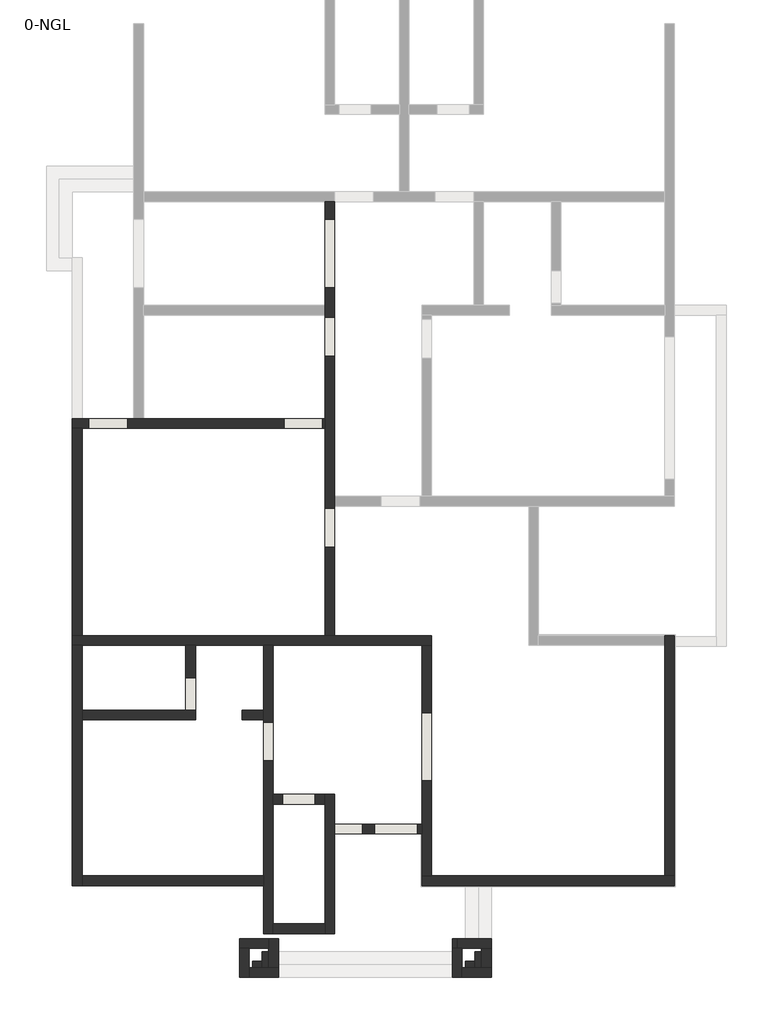
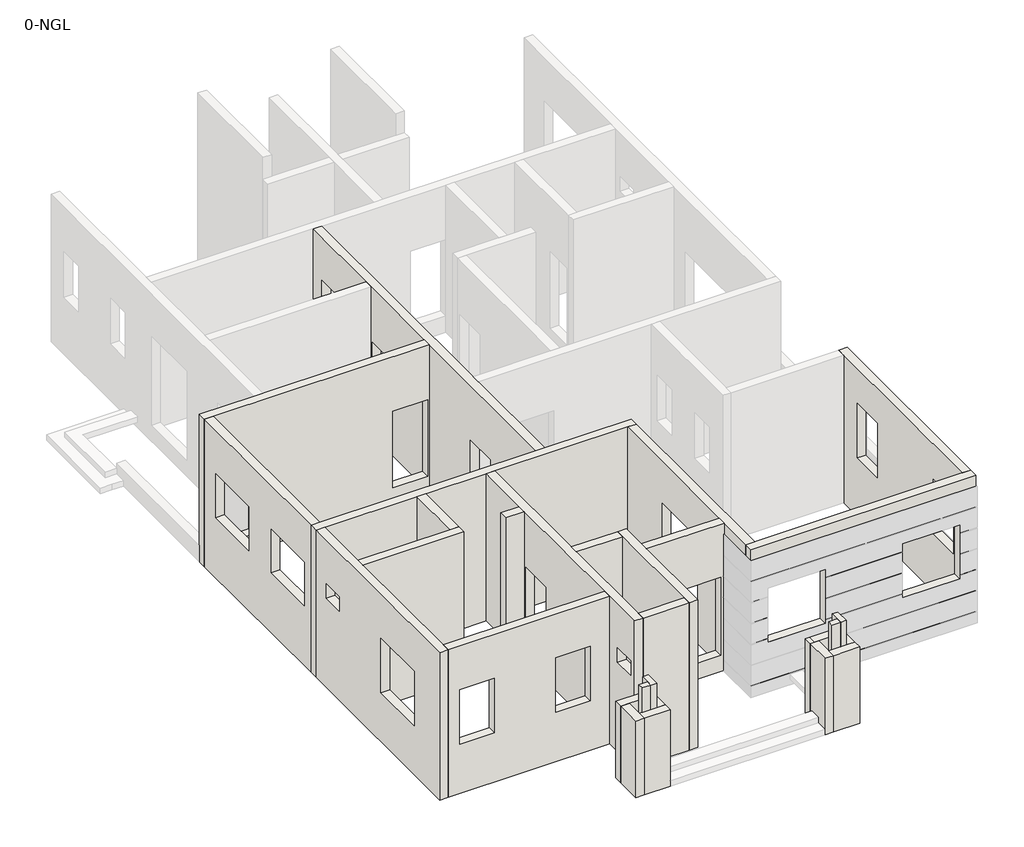
# One storey, part 1 of 2: 31 walls.
"""IFC4 building model written with IfcOpenShell, lengths in millimetres."""

from ifc_helpers import new_model, si_unit, frame, origin, origin_with_axes, place, context, project, spatial, polyline, outline, extrude, faceted_brep, element, save

model = new_model("IFC4")

# Units and contexts
model_context = context("Model", 3, world=origin())
ifc_project = project(units=[si_unit("LENGTHUNIT", "METRE", prefix="MILLI")], contexts=[model_context])

# Site, building, storey
site = spatial("IfcSite", under=ifc_project)
building = spatial("IfcBuilding", under=site)
storey = spatial("IfcBuildingStorey", under=building, Name="0-NGL", Elevation=0.0)

# Walls
placement = place(None, origin())
element("IfcWall", 1, ObjectType="150mm wall", at=placement, inside=storey, context=model_context, shape_type="Brep", body=[
    faceted_brep([(-1711.7953966, -12624.1929163, 0.0), (-1711.7953966, -12849.1929163, 0.0), (-1711.7953966, -12999.1929163, 0.0), (-1711.7953966, -12999.1929163, 2775.0), (-1711.7953966, -12849.1929163, 2775.0), (-1711.7953966, -12624.1929163, 2775.0), (-1561.7953966, -12624.1929163, 0.0), (-1561.7953966, -12624.1929163, 2775.0), (-1561.7953966, -12999.1929163, 2775.0), (-1561.7953966, -12999.1929163, 0.0)], [[[0, 1, 2, 3, 4, 5]], [[6, 7, 8, 9]], [[2, 1, 0, 6, 9]], [[5, 4, 3, 8, 7]], [[0, 5, 7, 6]], [[3, 2, 9, 8]]]),
])
element("IfcWall", 2, ObjectType="150mm wall", at=placement, inside=storey, context=model_context, shape_type="SweptSolid", body=[
    extrude(outline(polyline([(-1936.7953966, -12849.1929163), (-1711.7953966, -12849.1929163), (-1711.7953966, -12999.1929163), (-1936.7953966, -12999.1929163), (-1936.7953966, -12849.1929163)])), origin_with_axes(), (0.0, 0.0, 1.0), 2775.0),
])
element("IfcWall", 3, ObjectType="150mm wall", at=placement, inside=storey, context=model_context, shape_type="Brep", body=[
    faceted_brep([(3218.2046034, -12624.1929163, 0.0), (3218.2046034, -12849.1929163, 0.0), (3218.2046034, -12999.1929163, 0.0), (3218.2046034, -12999.1929163, 2775.0), (3218.2046034, -12849.1929163, 2775.0), (3218.2046034, -12624.1929163, 2775.0), (3368.2046034, -12624.1929163, 0.0), (3368.2046034, -12624.1929163, 2775.0), (3368.2046034, -12999.1929163, 2775.0), (3368.2046034, -12999.1929163, 0.0)], [[[0, 1, 2, 3, 4, 5]], [[6, 7, 8, 9]], [[2, 1, 0, 6, 9]], [[5, 4, 3, 8, 7]], [[0, 5, 7, 6]], [[3, 2, 9, 8]]]),
])
element("IfcWall", 4, ObjectType="150mm wall", at=placement, inside=storey, context=model_context, shape_type="SweptSolid", body=[
    extrude(outline(polyline([(2993.2046034, -12849.1929163), (3218.2046034, -12849.1929163), (3218.2046034, -12999.1929163), (2993.2046034, -12999.1929163), (2993.2046034, -12849.1929163)])), origin_with_axes(), (0.0, 0.0, 1.0), 2775.0),
])
element("IfcWall", 5, ObjectType="225 wall", at=placement, inside=storey, context=model_context, shape_type="Brep", body=[
    faceted_brep([(7838.2046034, -10871.6929163, 0.0), (7613.2046034, -10871.6929163, 0.0), (2213.2046034, -10871.6929163, 0.0), (1988.2046034, -10871.6929163, 0.0), (1988.2046034, -10871.6929163, 4050.0), (2213.2046034, -10871.6929163, 4050.0), (7613.2046034, -10871.6929163, 4050.0), (7838.2046034, -10871.6929163, 4050.0), (3913.2046034, -10871.6929163, 2850.0), (2413.2046034, -10871.6929163, 2850.0), (2413.2046034, -10871.6929163, 1350.0), (3913.2046034, -10871.6929163, 1350.0), (7413.2046034, -10871.6929163, 2850.0), (5913.2046034, -10871.6929163, 2850.0), (5913.2046034, -10871.6929163, 1350.0), (7413.2046034, -10871.6929163, 1350.0), (7838.2046034, -11096.6929163, 0.0), (7838.2046034, -11096.6929163, 4050.0), (1988.2046034, -11096.6929163, 4050.0), (1988.2046034, -11096.6929163, 0.0), (3913.2046034, -11096.6929163, 2850.0), (3913.2046034, -11096.6929163, 1350.0), (2413.2046034, -11096.6929163, 1350.0), (2413.2046034, -11096.6929163, 2850.0), (7413.2046034, -11096.6929163, 2850.0), (7413.2046034, -11096.6929163, 1350.0), (5913.2046034, -11096.6929163, 1350.0), (5913.2046034, -11096.6929163, 2850.0)], [[[0, 1, 2, 3, 4, 5, 6, 7], [8, 9, 10, 11], [12, 13, 14, 15]], [[16, 17, 18, 19], [20, 21, 22, 23], [24, 25, 26, 27]], [[3, 2, 1, 0, 16, 19]], [[7, 6, 5, 4, 18, 17]], [[0, 7, 17, 16]], [[4, 3, 19, 18]], [[21, 20, 8, 11]], [[22, 21, 11, 10]], [[23, 22, 10, 9]], [[20, 23, 9, 8]], [[25, 24, 12, 15]], [[26, 25, 15, 14]], [[27, 26, 14, 13]], [[24, 27, 13, 12]]]),
])
element("IfcWall", 6, ObjectType="225 wall", at=placement, inside=storey, context=model_context, shape_type="Brep", body=[
    faceted_brep([(-5886.7953966, -11096.6929163, 0.0), (-5886.7953966, -10871.6929163, 0.0), (-5886.7953966, -7259.1929163, 0.0), (-5886.7953966, -7034.1929163, 0.0), (-5886.7953966, -5534.1929163, 0.0), (-5886.7953966, -5534.1929163, 4050.0), (-5886.7953966, -7034.1929163, 4050.0), (-5886.7953966, -7259.1929163, 4050.0), (-5886.7953966, -10871.6929163, 4050.0), (-5886.7953966, -11096.6929163, 4050.0), (-5886.7953966, -6584.1929163, 2850.0), (-5886.7953966, -5984.1929163, 2850.0), (-5886.7953966, -5984.1929163, 2450.0), (-5886.7953966, -6584.1929163, 2450.0), (-5886.7953966, -8459.1929163, 2850.0), (-5886.7953966, -8459.1929163, 1350.0), (-5886.7953966, -9959.1929163, 1350.0), (-5886.7953966, -9959.1929163, 2850.0), (-6111.7953966, -11096.6929163, 0.0), (-6111.7953966, -11096.6929163, 4050.0), (-6111.7953966, -5534.1929163, 4050.0), (-6111.7953966, -5534.1929163, 0.0), (-6111.7953966, -6584.1929163, 2850.0), (-6111.7953966, -6584.1929163, 2450.0), (-6111.7953966, -5984.1929163, 2450.0), (-6111.7953966, -5984.1929163, 2850.0), (-6111.7953966, -8459.1929163, 2850.0), (-6111.7953966, -9959.1929163, 2850.0), (-6111.7953966, -9959.1929163, 1350.0), (-6111.7953966, -8459.1929163, 1350.0)], [[[0, 1, 2, 3, 4, 5, 6, 7, 8, 9], [10, 11, 12, 13], [14, 15, 16, 17]], [[18, 19, 20, 21], [22, 23, 24, 25], [26, 27, 28, 29]], [[4, 3, 2, 1, 0, 18, 21]], [[9, 8, 7, 6, 5, 20, 19]], [[5, 4, 21, 20]], [[0, 9, 19, 18]], [[23, 22, 10, 13]], [[24, 23, 13, 12]], [[25, 24, 12, 11]], [[22, 25, 11, 10]], [[15, 14, 26, 29]], [[16, 15, 29, 28]], [[17, 16, 28, 27]], [[14, 17, 27, 26]]]),
])
element("IfcWall", 7, ObjectType="225 wall", at=placement, inside=storey, context=model_context, shape_type="Brep", body=[
    faceted_brep([(-1461.7953966, -12209.1929163, 4050.0), (-1461.7953966, -12209.1929163, 0.0), (-1461.7953966, -11984.1929163, 0.0), (-1461.7953966, -9209.1929163, 0.0), (-1461.7953966, -8984.1929163, 0.0), (-1461.7953966, -5534.1929163, 0.0), (-1461.7953966, -5534.1929163, 4050.0), (-1461.7953966, -8984.1929163, 4050.0), (-1461.7953966, -9209.1929163, 4050.0), (-1461.7953966, -11984.1929163, 4050.0), (-1461.7953966, -7309.1929163, 450.0), (-1461.7953966, -8209.1929163, 450.0), (-1461.7953966, -8209.1929163, 2550.0), (-1461.7953966, -7309.1929163, 2550.0), (-1461.7953966, -11444.1929163, 2850.0), (-1461.7953966, -11444.1929163, 2450.0), (-1461.7953966, -12044.1929163, 2450.0), (-1461.7953966, -12044.1929163, 2850.0), (-1686.7953966, -12209.1929163, 0.0), (-1686.7953966, -12209.1929163, 4050.0), (-1686.7953966, -11096.6929163, 4050.0), (-1686.7953966, -10871.6929163, 4050.0), (-1686.7953966, -7259.1929163, 4050.0), (-1686.7953966, -7034.1929163, 4050.0), (-1686.7953966, -5534.1929163, 4050.0), (-1686.7953966, -5534.1929163, 0.0), (-1686.7953966, -7034.1929163, 0.0), (-1686.7953966, -7259.1929163, 0.0), (-1686.7953966, -10871.6929163, 0.0), (-1686.7953966, -11096.6929163, 0.0), (-1686.7953966, -7309.1929163, 450.0), (-1686.7953966, -7309.1929163, 2550.0), (-1686.7953966, -8209.1929163, 2550.0), (-1686.7953966, -8209.1929163, 450.0), (-1686.7953966, -11444.1929163, 2850.0), (-1686.7953966, -12044.1929163, 2850.0), (-1686.7953966, -12044.1929163, 2450.0), (-1686.7953966, -11444.1929163, 2450.0)], [[[0, 1, 2, 3, 4, 5, 6, 7, 8, 9], [10, 11, 12, 13], [14, 15, 16, 17]], [[18, 19, 20, 21, 22, 23, 24, 25, 26, 27, 28, 29], [30, 31, 32, 33], [34, 35, 36, 37]], [[5, 4, 3, 2, 1, 18, 29, 28, 27, 26, 25]], [[0, 9, 8, 7, 6, 24, 23, 22, 21, 20, 19]], [[6, 5, 25, 24]], [[31, 30, 10, 13]], [[32, 31, 13, 12]], [[33, 32, 12, 11]], [[30, 33, 11, 10]], [[15, 14, 34, 37]], [[16, 15, 37, 36]], [[17, 16, 36, 35]], [[14, 17, 35, 34]], [[0, 19, 18, 1]]]),
])
element("IfcWall", 8, ObjectType="225 wall", at=placement, inside=storey, context=model_context, shape_type="Brep", body=[
    faceted_brep([(-6111.7953966, -509.1929163, 4050.0), (-6111.7953966, -509.1929163, 0.0), (-5886.7953966, -509.1929163, 0.0), (-261.7953966, -509.1929163, 0.0), (-261.7953966, -509.1929163, 4050.0), (-5886.7953966, -509.1929163, 4050.0), (-4836.7953966, -509.1929163, 450.0), (-5736.7953966, -509.1929163, 450.0), (-5736.7953966, -509.1929163, 2550.0), (-4836.7953966, -509.1929163, 2550.0), (-311.7953966, -509.1929163, 450.0), (-1211.7953966, -509.1929163, 450.0), (-1211.7953966, -509.1929163, 2550.0), (-311.7953966, -509.1929163, 2550.0), (-6111.7953966, -284.1929163, 0.0), (-6111.7953966, -284.1929163, 450.0), (-6111.7953966, -284.1929163, 3450.0), (-6111.7953966, -284.1929163, 4042.0), (-6111.7953966, -284.1929163, 4050.0), (-4686.7953966, -284.1929163, 4050.0), (-4461.7953966, -284.1929163, 4050.0), (-261.7953966, -284.1929163, 4050.0), (-261.7953966, -284.1929163, 0.0), (-4461.7953966, -284.1929163, 0.0), (-4686.7953966, -284.1929163, 0.0), (-5886.7953966, -284.1929163, 0.0), (-4836.7953966, -284.1929163, 450.0), (-4836.7953966, -284.1929163, 2550.0), (-5736.7953966, -284.1929163, 2550.0), (-5736.7953966, -284.1929163, 450.0), (-311.7953966, -284.1929163, 450.0), (-311.7953966, -284.1929163, 2550.0), (-1211.7953966, -284.1929163, 2550.0), (-1211.7953966, -284.1929163, 450.0)], [[[0, 1, 2, 3, 4, 5], [6, 7, 8, 9], [10, 11, 12, 13]], [[14, 15, 16, 17, 18, 19, 20, 21, 22, 23, 24, 25], [26, 27, 28, 29], [30, 31, 32, 33]], [[3, 2, 1, 14, 25, 24, 23, 22]], [[0, 5, 4, 21, 20, 19, 18]], [[4, 3, 22, 21]], [[27, 26, 6, 9]], [[28, 27, 9, 8]], [[29, 28, 8, 7]], [[26, 29, 7, 6]], [[31, 30, 10, 13]], [[32, 31, 13, 12]], [[33, 32, 12, 11]], [[30, 33, 11, 10]], [[0, 18, 17, 16, 15, 14, 1]]]),
])
element("IfcWall", 9, ObjectType="225 wall", at=placement, inside=storey, context=model_context, shape_type="Brep", body=[
    faceted_brep([(7838.2046034, -10871.6929163, 0.0), (7838.2046034, -5559.1929163, 0.0), (7838.2046034, -5334.1929163, 0.0), (7838.2046034, -5309.1929163, 0.0), (7838.2046034, -5309.1929163, 3450.0), (7838.2046034, -5309.1929163, 4050.0), (7838.2046034, -10871.6929163, 4050.0), (7838.2046034, -9571.6929163, 3090.0), (7838.2046034, -9571.6929163, 1590.0), (7838.2046034, -10471.6929163, 1590.0), (7838.2046034, -10471.6929163, 3090.0), (7838.2046034, -6134.1929163, 3090.0), (7838.2046034, -6134.1929163, 1590.0), (7838.2046034, -7034.1929163, 1590.0), (7838.2046034, -7034.1929163, 3090.0), (7613.2046034, -10871.6929163, 0.0), (7613.2046034, -10871.6929163, 4050.0), (7613.2046034, -5534.1929163, 4050.0), (7613.2046034, -5309.1929163, 4050.0), (7613.2046034, -5309.1929163, 0.0), (7613.2046034, -5534.1929163, 0.0), (7613.2046034, -9571.6929163, 3090.0), (7613.2046034, -10471.6929163, 3090.0), (7613.2046034, -10471.6929163, 1590.0), (7613.2046034, -9571.6929163, 1590.0), (7613.2046034, -6134.1929163, 3090.0), (7613.2046034, -7034.1929163, 3090.0), (7613.2046034, -7034.1929163, 1590.0), (7613.2046034, -6134.1929163, 1590.0)], [[[0, 1, 2, 3, 4, 5, 6], [7, 8, 9, 10], [11, 12, 13, 14]], [[15, 16, 17, 18, 19, 20], [21, 22, 23, 24], [25, 26, 27, 28]], [[3, 2, 1, 0, 15, 20, 19]], [[6, 5, 18, 17, 16]], [[0, 6, 16, 15]], [[8, 7, 21, 24]], [[9, 8, 24, 23]], [[10, 9, 23, 22]], [[7, 10, 22, 21]], [[12, 11, 25, 28]], [[13, 12, 28, 27]], [[14, 13, 27, 26]], [[11, 14, 26, 25]], [[3, 19, 18, 5, 4]]]),
])
element("IfcWall", 10, ObjectType="225 wall", at=placement, inside=storey, context=model_context, shape_type="Brep", body=[
    faceted_brep([(-6111.7953966, -5534.1929163, 0.0), (-5886.7953966, -5534.1929163, 0.0), (-3486.7953966, -5534.1929163, 0.0), (-3261.7953966, -5534.1929163, 0.0), (-1686.7953966, -5534.1929163, 0.0), (-1461.7953966, -5534.1929163, 0.0), (1988.2046034, -5534.1929163, 0.0), (2213.2046034, -5534.1929163, 0.0), (2213.2046034, -5534.1929163, 4050.0), (1988.2046034, -5534.1929163, 4050.0), (-1461.7953966, -5534.1929163, 4050.0), (-1686.7953966, -5534.1929163, 4050.0), (-3261.7953966, -5534.1929163, 4050.0), (-3486.7953966, -5534.1929163, 4050.0), (-5886.7953966, -5534.1929163, 4050.0), (-6111.7953966, -5534.1929163, 4050.0), (-6111.7953966, -5309.1929163, 0.0), (-6111.7953966, -5309.1929163, 4050.0), (-5886.7953966, -5309.1929163, 4050.0), (-261.7953966, -5309.1929163, 4050.0), (-36.7953966, -5309.1929163, 4050.0), (2213.2046034, -5309.1929163, 4050.0), (2213.2046034, -5309.1929163, 0.0), (-36.7953966, -5309.1929163, 0.0), (-261.7953966, -5309.1929163, 0.0), (-5886.7953966, -5309.1929163, 0.0)], [[[0, 1, 2, 3, 4, 5, 6, 7, 8, 9, 10, 11, 12, 13, 14, 15]], [[16, 17, 18, 19, 20, 21, 22, 23, 24, 25]], [[7, 6, 5, 4, 3, 2, 1, 0, 16, 25, 24, 23, 22]], [[15, 14, 13, 12, 11, 10, 9, 8, 21, 20, 19, 18, 17]], [[0, 15, 17, 16]], [[8, 7, 22, 21]]]),
])
element("IfcWall", 11, ObjectType="225 wall", at=placement, inside=storey, context=model_context, shape_type="SweptSolid", body=[
    extrude(outline(polyline([(-5309.1929163, 0.0), (-5309.1929163, 4050.0), (-509.1929163, 4050.0), (-509.1929163, 0.0), (-5309.1929163, 0.0)]), holes=[polyline([(-1009.1929163, 2850.0), (-2509.1929163, 2850.0), (-2509.1929163, 1650.0), (-1009.1929163, 1650.0), (-1009.1929163, 2850.0)]), polyline([(-3509.1929163, 2850.0), (-5009.1929163, 2850.0), (-5009.1929163, 1650.0), (-3509.1929163, 1650.0), (-3509.1929163, 2850.0)])]), frame((-6111.7953966, 0.0, 0.0), z_axis=(1.0, 0.0, 0.0), x_axis=(0.0, 1.0, 0.0)), (0.0, 0.0, 1.0), 225.0),
])
element("IfcWall", 12, ObjectType="225 wall", at=placement, inside=storey, context=model_context, shape_type="Brep", body=[
    faceted_brep([(-5886.7953966, -7259.1929163, 0.0), (-3261.7953966, -7259.1929163, 0.0), (-3261.7953966, -7259.1929163, 4050.0), (-5886.7953966, -7259.1929163, 4050.0), (-5886.7953966, -7034.1929163, 0.0), (-5886.7953966, -7034.1929163, 4050.0), (-3486.7953966, -7034.1929163, 4050.0), (-3261.7953966, -7034.1929163, 4050.0), (-3261.7953966, -7034.1929163, 2550.0), (-3261.7953966, -7034.1929163, 450.0), (-3261.7953966, -7034.1929163, 0.0), (-3486.7953966, -7034.1929163, 0.0)], [[[0, 1, 2, 3]], [[4, 5, 6, 7, 8, 9, 10, 11]], [[1, 0, 4, 11, 10]], [[2, 1, 10, 9, 8, 7]], [[3, 2, 7, 6, 5]], [[0, 3, 5, 4]]]),
])
element("IfcWall", 13, ObjectType="225 wall", at=placement, inside=storey, context=model_context, shape_type="SweptSolid", body=[
    extrude(outline(polyline([(0.0, -5886.7953966), (0.0, -1686.7953966), (4050.0, -1686.7953966), (4050.0, -5886.7953966), (0.0, -5886.7953966)]), holes=[polyline([(2850.0, -2186.7953966), (1350.0, -2186.7953966), (1350.0, -3086.7953966), (2850.0, -3086.7953966), (2850.0, -2186.7953966)]), polyline([(2850.0, -4686.7953966), (1350.0, -4686.7953966), (1350.0, -5586.7953966), (2850.0, -5586.7953966), (2850.0, -4686.7953966)])]), frame((0.0, -11096.6929163, 0.0), z_axis=(0.0, 1.0, 0.0), x_axis=(0.0, 0.0, 1.0)), (0.0, 0.0, 1.0), 225.0),
])
element("IfcWall", 14, ObjectType="225 wall", at=placement, inside=storey, context=model_context, shape_type="Brep", body=[
    faceted_brep([(2213.2046034, -10871.6929163, 0.0), (2213.2046034, -5534.1929163, 0.0), (2213.2046034, -5534.1929163, 4050.0), (2213.2046034, -10871.6929163, 4050.0), (2213.2046034, -7091.6929163, 450.0), (2213.2046034, -8671.6929163, 450.0), (2213.2046034, -8671.6929163, 2890.0), (2213.2046034, -7091.6929163, 2890.0), (1988.2046034, -10871.6929163, 0.0), (1988.2046034, -10871.6929163, 4050.0), (1988.2046034, -9896.6929163, 4050.0), (1988.2046034, -9671.6929163, 4050.0), (1988.2046034, -5534.1929163, 4050.0), (1988.2046034, -5534.1929163, 0.0), (1988.2046034, -9671.6929163, 0.0), (1988.2046034, -9896.6929163, 0.0), (1988.2046034, -7091.6929163, 450.0), (1988.2046034, -7091.6929163, 2890.0), (1988.2046034, -8671.6929163, 2890.0), (1988.2046034, -8671.6929163, 450.0)], [[[0, 1, 2, 3], [4, 5, 6, 7]], [[8, 9, 10, 11, 12, 13, 14, 15], [16, 17, 18, 19]], [[1, 0, 8, 15, 14, 13]], [[3, 2, 12, 11, 10, 9]], [[0, 3, 9, 8]], [[17, 16, 4, 7]], [[18, 17, 7, 6]], [[19, 18, 6, 5]], [[16, 19, 5, 4]], [[2, 1, 13, 12]]]),
])
element("IfcWall", 15, ObjectType="225 wall", at=placement, inside=storey, context=model_context, shape_type="Brep", body=[
    faceted_brep([(-36.7953966, -5309.1929163, 0.0), (-36.7953966, -2309.1929163, 0.0), (-36.7953966, -2084.1929163, 0.0), (-36.7953966, 4740.8070837, 0.0), (-36.7953966, 4740.8070837, 450.0), (-36.7953966, 4740.8070837, 2550.0), (-36.7953966, 4740.8070837, 4050.0), (-36.7953966, -2084.1929163, 4050.0), (-36.7953966, -2309.1929163, 4050.0), (-36.7953966, -5309.1929163, 4050.0), (-36.7953966, -2359.1929163, 450.0), (-36.7953966, -3259.1929163, 450.0), (-36.7953966, -3259.1929163, 2550.0), (-36.7953966, -2359.1929163, 2550.0), (-36.7953966, 4330.8070837, 450.0), (-36.7953966, 2750.8070837, 450.0), (-36.7953966, 2750.8070837, 2890.0), (-36.7953966, 4330.8070837, 2890.0), (-36.7953966, 2065.8070837, 450.0), (-36.7953966, 1165.8070837, 450.0), (-36.7953966, 1165.8070837, 2550.0), (-36.7953966, 2065.8070837, 2550.0), (-261.7953966, -5309.1929163, 0.0), (-261.7953966, -5309.1929163, 4050.0), (-261.7953966, -509.1929163, 4050.0), (-261.7953966, -284.1929163, 4050.0), (-261.7953966, 2115.8070837, 4050.0), (-261.7953966, 2340.8070837, 4050.0), (-261.7953966, 4740.8070837, 4050.0), (-261.7953966, 4740.8070837, 0.0), (-261.7953966, 2340.8070837, 0.0), (-261.7953966, 2115.8070837, 0.0), (-261.7953966, -284.1929163, 0.0), (-261.7953966, -509.1929163, 0.0), (-261.7953966, -2359.1929163, 450.0), (-261.7953966, -2359.1929163, 2550.0), (-261.7953966, -3259.1929163, 2550.0), (-261.7953966, -3259.1929163, 450.0), (-261.7953966, 4330.8070837, 450.0), (-261.7953966, 4330.8070837, 2890.0), (-261.7953966, 2750.8070837, 2890.0), (-261.7953966, 2750.8070837, 450.0), (-261.7953966, 2065.8070837, 450.0), (-261.7953966, 2065.8070837, 2550.0), (-261.7953966, 1165.8070837, 2550.0), (-261.7953966, 1165.8070837, 450.0)], [[[0, 1, 2, 3, 4, 5, 6, 7, 8, 9], [10, 11, 12, 13], [14, 15, 16, 17], [18, 19, 20, 21]], [[22, 23, 24, 25, 26, 27, 28, 29, 30, 31, 32, 33], [34, 35, 36, 37], [38, 39, 40, 41], [42, 43, 44, 45]], [[3, 2, 1, 0, 22, 33, 32, 31, 30, 29]], [[9, 8, 7, 6, 28, 27, 26, 25, 24, 23]], [[6, 5, 4, 3, 29, 28]], [[0, 9, 23, 22]], [[35, 34, 10, 13]], [[36, 35, 13, 12]], [[37, 36, 12, 11]], [[34, 37, 11, 10]], [[39, 38, 14, 17]], [[40, 39, 17, 16]], [[41, 40, 16, 15]], [[38, 41, 15, 14]], [[43, 42, 18, 21]], [[44, 43, 21, 20]], [[45, 44, 20, 19]], [[42, 45, 19, 18]]]),
])
element("IfcWall", 16, ObjectType="225 wall", at=placement, inside=storey, context=model_context, shape_type="Brep", body=[
    faceted_brep([(-36.7953966, -12209.1929163, 0.0), (-36.7953966, -9896.6929163, 0.0), (-36.7953966, -9671.6929163, 0.0), (-36.7953966, -8984.1929163, 0.0), (-36.7953966, -8984.1929163, 4050.0), (-36.7953966, -9671.6929163, 4050.0), (-36.7953966, -9896.6929163, 4050.0), (-36.7953966, -12209.1929163, 4050.0), (-261.7953966, -8984.1929163, 0.0), (-261.7953966, -9209.1929163, 0.0), (-261.7953966, -11984.1929163, 0.0), (-261.7953966, -12209.1929163, 0.0), (-261.7953966, -12209.1929163, 4050.0), (-261.7953966, -11984.1929163, 4050.0), (-261.7953966, -9209.1929163, 4050.0), (-261.7953966, -8984.1929163, 4050.0)], [[[0, 1, 2, 3, 4, 5, 6, 7]], [[8, 9, 10, 11, 12, 13, 14, 15]], [[3, 2, 1, 0, 11, 10, 9, 8]], [[7, 6, 5, 4, 15, 14, 13, 12]], [[4, 3, 8, 15]], [[0, 7, 12, 11]]]),
])
element("IfcWall", 17, ObjectType="225 wall", at=placement, inside=storey, context=model_context, shape_type="SweptSolid", body=[
    extrude(outline(polyline([(0.0, -261.7953966), (4050.0, -261.7953966), (4050.0, -1461.7953966), (0.0, -1461.7953966), (0.0, -261.7953966)]), holes=[polyline([(450.0, -1236.7953966), (2550.0, -1236.7953966), (2550.0, -486.7953966), (450.0, -486.7953966), (450.0, -1236.7953966)])]), frame((0.0, -9209.1929163, 0.0), z_axis=(0.0, 1.0, 0.0), x_axis=(0.0, 0.0, 1.0)), (0.0, 0.0, 1.0), 225.0),
])
element("IfcWall", 18, ObjectType="225 wall", at=placement, inside=storey, context=model_context, shape_type="SweptSolid", body=[
    extrude(outline(polyline([(-1461.7953966, -11984.1929163), (-261.7953966, -11984.1929163), (-261.7953966, -12209.1929163), (-1461.7953966, -12209.1929163), (-1461.7953966, -11984.1929163)])), origin_with_axes(), (0.0, 0.0, 1.0), 4050.0),
])
element("IfcWall", 19, ObjectType="225 wall", at=placement, inside=storey, context=model_context, shape_type="SweptSolid", body=[
    extrude(outline(polyline([(0.0, -36.7953966), (0.0, 1988.2046034), (4050.0, 1988.2046034), (4050.0, -36.7953966), (2275.0, -36.7953966), (2275.0, 613.2046034), (1025.0, 613.2046034), (1025.0, -36.7953966), (0.0, -36.7953966)]), holes=[polyline([(450.0, 888.2046034), (2595.0, 888.2046034), (2595.0, 1888.2046034), (450.0, 1888.2046034), (450.0, 888.2046034)])]), frame((0.0, -9896.6929163, 0.0), z_axis=(0.0, 1.0, 0.0), x_axis=(0.0, 0.0, 1.0)), (0.0, 0.0, 1.0), 225.0),
])
element("IfcWall", 20, ObjectType="225 wall", at=placement, inside=storey, context=model_context, shape_type="SweptSolid", body=[
    extrude(outline(polyline([(-6284.1929163, 2550.0), (-7034.1929163, 2550.0), (-7034.1929163, 4050.0), (-5534.1929163, 4050.0), (-5534.1929163, 0.0), (-7034.1929163, 0.0), (-7034.1929163, 450.0), (-6284.1929163, 450.0), (-6284.1929163, 2550.0)])), frame((-3486.7953966, 0.0, 0.0), z_axis=(1.0, 0.0, 0.0), x_axis=(0.0, 1.0, 0.0)), (0.0, 0.0, 1.0), 225.0),
])
element("IfcWall", 21, ObjectType="225 wall", at=placement, inside=storey, context=model_context, shape_type="SweptSolid", body=[
    extrude(outline(polyline([(-1686.7953966, -7259.1929163), (-2174.2953966, -7259.1929163), (-2174.2953966, -7034.1929163), (-1686.7953966, -7034.1929163), (-1686.7953966, -7259.1929163)])), origin_with_axes(), (0.0, 0.0, 1.0), 4050.0),
])
element("IfcWall", 22, ObjectType="225 wall", at=placement, inside=storey, context=model_context, shape_type="Brep", body=[
    faceted_brep([(-2236.7953966, -12549.1929163, 0.0), (-2011.7953966, -12549.1929163, 0.0), (-1561.7953966, -12549.1929163, 0.0), (-1561.7953966, -12549.1929163, 2100.0), (-2011.7953966, -12549.1929163, 2100.0), (-2236.7953966, -12549.1929163, 2100.0), (-2236.7953966, -12324.1929163, 0.0), (-2236.7953966, -12324.1929163, 2100.0), (-1561.7953966, -12324.1929163, 2100.0), (-1561.7953966, -12324.1929163, 0.0)], [[[0, 1, 2, 3, 4, 5]], [[6, 7, 8, 9]], [[2, 1, 0, 6, 9]], [[5, 4, 3, 8, 7]], [[0, 5, 7, 6]], [[3, 2, 9, 8]]]),
])
element("IfcWall", 23, ObjectType="225 wall", at=placement, inside=storey, context=model_context, shape_type="Brep", body=[
    faceted_brep([(-2011.7953966, -13224.1929163, 0.0), (-2011.7953966, -12999.1929163, 0.0), (-2011.7953966, -12549.1929163, 0.0), (-2011.7953966, -12549.1929163, 2100.0), (-2011.7953966, -12999.1929163, 2100.0), (-2011.7953966, -13224.1929163, 2100.0), (-2236.7953966, -13224.1929163, 0.0), (-2236.7953966, -13224.1929163, 2100.0), (-2236.7953966, -12549.1929163, 2100.0), (-2236.7953966, -12549.1929163, 0.0)], [[[0, 1, 2, 3, 4, 5]], [[6, 7, 8, 9]], [[2, 1, 0, 6, 9]], [[5, 4, 3, 8, 7]], [[0, 5, 7, 6]], [[3, 2, 9, 8]]]),
])
element("IfcWall", 24, ObjectType="225 wall", at=placement, inside=storey, context=model_context, shape_type="Brep", body=[
    faceted_brep([(-1336.7953966, -12999.1929163, 0.0), (-1561.7953966, -12999.1929163, 0.0), (-2011.7953966, -12999.1929163, 0.0), (-2011.7953966, -12999.1929163, 2100.0), (-1561.7953966, -12999.1929163, 2100.0), (-1336.7953966, -12999.1929163, 2100.0), (-1336.7953966, -13224.1929163, 0.0), (-1336.7953966, -13224.1929163, 2100.0), (-2011.7953966, -13224.1929163, 2100.0), (-2011.7953966, -13224.1929163, 0.0)], [[[0, 1, 2, 3, 4, 5]], [[6, 7, 8, 9]], [[2, 1, 0, 6, 9]], [[5, 4, 3, 8, 7]], [[0, 5, 7, 6]], [[3, 2, 9, 8]]]),
])
element("IfcWall", 25, ObjectType="225 wall", at=placement, inside=storey, context=model_context, shape_type="Brep", body=[
    faceted_brep([(-1561.7953966, -12324.1929163, 0.0), (-1561.7953966, -12549.1929163, 0.0), (-1561.7953966, -12999.1929163, 0.0), (-1561.7953966, -12999.1929163, 2100.0), (-1561.7953966, -12549.1929163, 2100.0), (-1561.7953966, -12324.1929163, 2100.0), (-1336.7953966, -12324.1929163, 0.0), (-1336.7953966, -12324.1929163, 2100.0), (-1336.7953966, -12999.1929163, 2100.0), (-1336.7953966, -12999.1929163, 0.0)], [[[0, 1, 2, 3, 4, 5]], [[6, 7, 8, 9]], [[2, 1, 0, 6, 9]], [[5, 4, 3, 8, 7]], [[0, 5, 7, 6]], [[3, 2, 9, 8]]]),
])
element("IfcWall", 26, ObjectType="225 wall", at=placement, inside=storey, context=model_context, shape_type="Brep", body=[
    faceted_brep([(2805.7046034, -12549.1929163, 0.0), (2918.2046034, -12549.1929163, 0.0), (3368.2046034, -12549.1929163, 0.0), (3593.2046034, -12549.1929163, 0.0), (3593.2046034, -12549.1929163, 2100.0), (3368.2046034, -12549.1929163, 2100.0), (2918.2046034, -12549.1929163, 2100.0), (2805.7046034, -12549.1929163, 2100.0), (2805.7046034, -12324.1929163, 0.0), (2805.7046034, -12324.1929163, 2100.0), (3593.2046034, -12324.1929163, 2100.0), (3593.2046034, -12324.1929163, 0.0)], [[[0, 1, 2, 3, 4, 5, 6, 7]], [[8, 9, 10, 11]], [[3, 2, 1, 0, 8, 11]], [[7, 6, 5, 4, 10, 9]], [[0, 7, 9, 8]], [[4, 3, 11, 10]]]),
])
element("IfcWall", 27, ObjectType="225 wall", at=placement, inside=storey, context=model_context, shape_type="Brep", body=[
    faceted_brep([(2805.7046034, -12549.1929163, 0.0), (2918.2046034, -12549.1929163, 0.0), (3368.2046034, -12549.1929163, 0.0), (3593.2046034, -12549.1929163, 0.0), (3593.2046034, -12549.1929163, 2100.0), (3368.2046034, -12549.1929163, 2100.0), (2918.2046034, -12549.1929163, 2100.0), (2805.7046034, -12549.1929163, 2100.0), (2805.7046034, -12324.1929163, 0.0), (2805.7046034, -12324.1929163, 2100.0), (3593.2046034, -12324.1929163, 2100.0), (3593.2046034, -12324.1929163, 0.0)], [[[0, 1, 2, 3, 4, 5, 6, 7]], [[8, 9, 10, 11]], [[3, 2, 1, 0, 8, 11]], [[7, 6, 5, 4, 10, 9]], [[0, 7, 9, 8]], [[4, 3, 11, 10]]]),
])
element("IfcWall", 28, ObjectType="225 wall", at=placement, inside=storey, context=model_context, shape_type="Brep", body=[
    faceted_brep([(2693.2046034, -12549.1929163, 0.0), (2918.2046034, -12549.1929163, 0.0), (3368.2046034, -12549.1929163, 0.0), (3368.2046034, -12549.1929163, 2100.0), (2918.2046034, -12549.1929163, 2100.0), (2693.2046034, -12549.1929163, 2100.0), (2693.2046034, -12324.1929163, 0.0), (2693.2046034, -12324.1929163, 2100.0), (3368.2046034, -12324.1929163, 2100.0), (3368.2046034, -12324.1929163, 0.0)], [[[0, 1, 2, 3, 4, 5]], [[6, 7, 8, 9]], [[2, 1, 0, 6, 9]], [[5, 4, 3, 8, 7]], [[0, 5, 7, 6]], [[3, 2, 9, 8]]]),
])
element("IfcWall", 29, ObjectType="225 wall", at=placement, inside=storey, context=model_context, shape_type="Brep", body=[
    faceted_brep([(2918.2046034, -13224.1929163, 0.0), (2918.2046034, -12999.1929163, 0.0), (2918.2046034, -12549.1929163, 0.0), (2918.2046034, -12549.1929163, 2100.0), (2918.2046034, -12999.1929163, 2100.0), (2918.2046034, -13224.1929163, 2100.0), (2693.2046034, -13224.1929163, 0.0), (2693.2046034, -13224.1929163, 2100.0), (2693.2046034, -12549.1929163, 2100.0), (2693.2046034, -12549.1929163, 0.0), (2805.7046034, -12549.1929163, 0.0), (2805.7046034, -12549.1929163, 2100.0)], [[[0, 1, 2, 3, 4, 5]], [[6, 7, 8, 9]], [[2, 1, 0, 6, 9, 10]], [[5, 4, 3, 11, 8, 7]], [[0, 5, 7, 6]], [[3, 2, 10, 9, 8, 11]]]),
])
element("IfcWall", 30, ObjectType="225 wall", at=placement, inside=storey, context=model_context, shape_type="Brep", body=[
    faceted_brep([(3593.2046034, -12999.1929163, 0.0), (3368.2046034, -12999.1929163, 0.0), (2918.2046034, -12999.1929163, 0.0), (2918.2046034, -12999.1929163, 2100.0), (3368.2046034, -12999.1929163, 2100.0), (3593.2046034, -12999.1929163, 2100.0), (3593.2046034, -13224.1929163, 0.0), (3593.2046034, -13224.1929163, 2100.0), (2918.2046034, -13224.1929163, 2100.0), (2918.2046034, -13224.1929163, 0.0)], [[[0, 1, 2, 3, 4, 5]], [[6, 7, 8, 9]], [[2, 1, 0, 6, 9]], [[5, 4, 3, 8, 7]], [[0, 5, 7, 6]], [[3, 2, 9, 8]]]),
])
element("IfcWall", 31, ObjectType="225 wall", at=placement, inside=storey, context=model_context, shape_type="SweptSolid", body=[
    extrude(outline(polyline([(3368.2046034, -12999.1929163), (3368.2046034, -12549.1929163), (3593.2046034, -12549.1929163), (3593.2046034, -12999.1929163), (3368.2046034, -12999.1929163)])), origin_with_axes(), (0.0, 0.0, 1.0), 2100.0),
])

save(model, "model.ifc")

# Revit data of these elements
# Type "150mm wall"
#   Layers, outside or top first: 150 mm "Concrete, Cast In Situ" (function 1)
# Type "225 wall"
#   Layers, outside or top first: 225 mm "Concrete, Cast In Situ" (function 1)
# Elements 1, 2, 3, 4 (IfcWall, "150mm wall")
#   Top Offset = -675 mm
#   Base Offset = 0 mm
#   wall height = 2775 mm
#   Phase Created = New Construction
#   Base Constraint = 0-NGL
#   Top Constraint = 2-CEILING
#   Materials on its faces: "Concrete, Cast In Situ"
# Elements 5, 6, 7, 8, 9, 10, 11, 12, 13, 14, 15, 16, 17, 18, 19, 20, 21 (IfcWall, "225 wall")
#   Top Offset = 0 mm
#   Base Offset = 0 mm
#   wall height = 4050 mm
#   Phase Created = New Construction
#   Base Constraint = 0-NGL
#   Top Constraint = 3-ROOF
#   Materials on its faces: "Concrete, Cast In Situ"
# Elements 22, 23, 24, 25, 26, 27, 28, 29, 30, 31 (IfcWall, "225 wall")
#   Top Offset = 0 mm
#   Base Offset = 0 mm
#   Unconnected Height = 2100 mm
#   wall height = 2100 mm
#   Phase Created = New Construction
#   Base Constraint = 0-NGL
#   Materials on its faces: "Concrete, Cast In Situ"
# Materials
#   "Concrete, Cast In Situ": class "Concrete", colour RGB 191 178 173, transparency 0, Description = "physical material", Cost = 0
